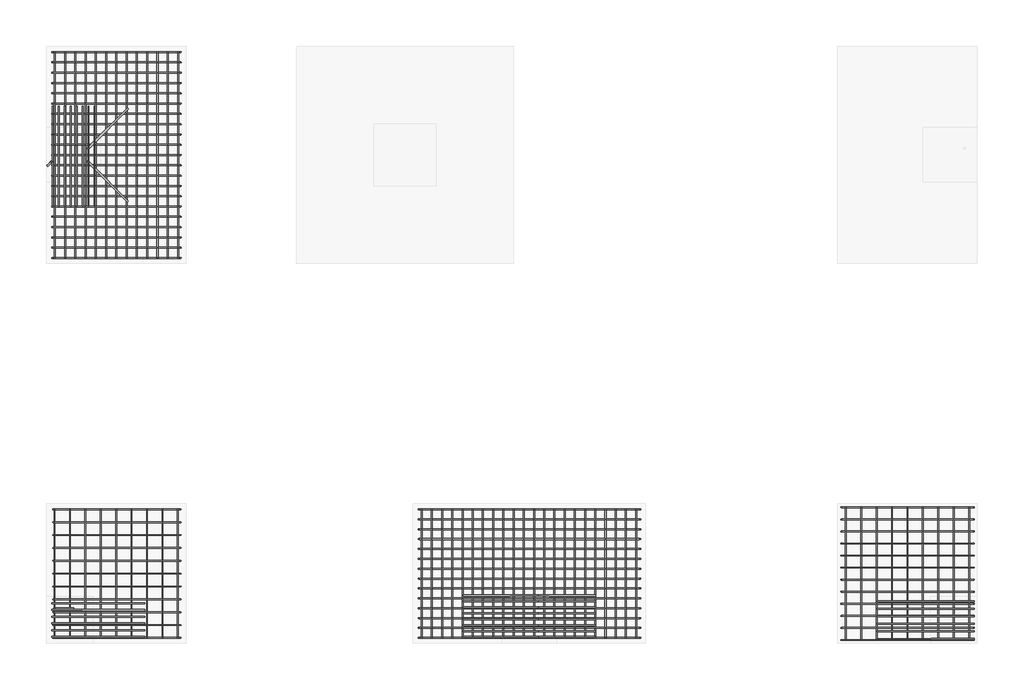
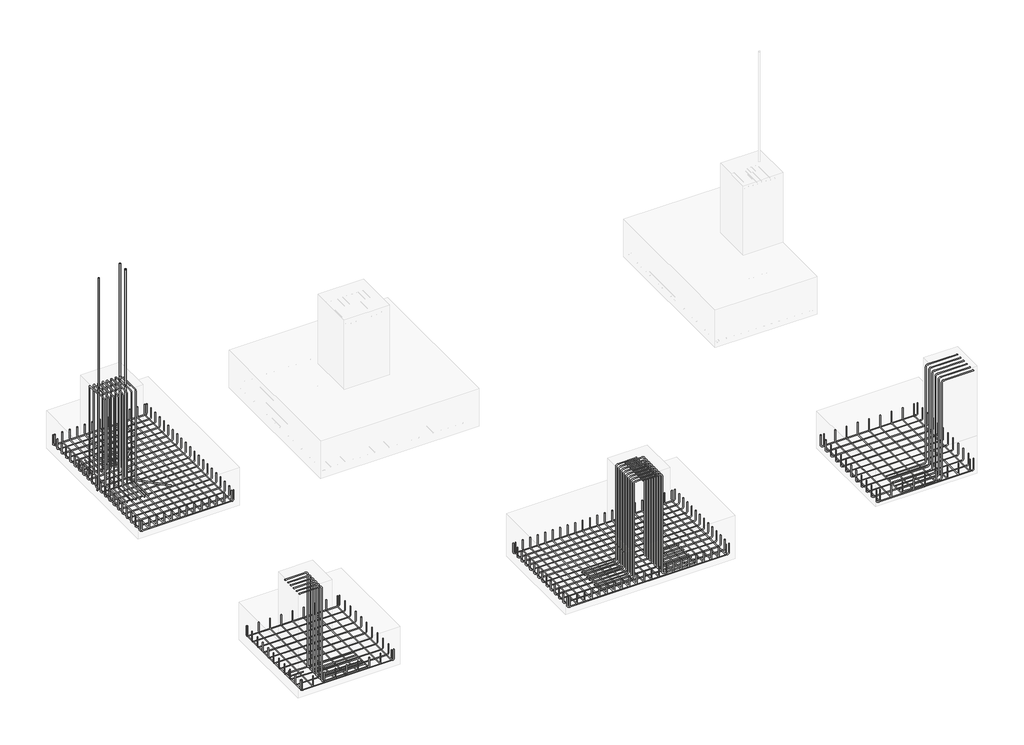
# One storey, part 2 of 6: 18 reinforcing bars.
"""IFC4 building model written with IfcOpenShell, lengths in millimetres."""

from ifc_helpers import new_model, si_unit, point, frame, origin, place, context, project, spatial, polyline, circle_curve, trimmed, segment, composite_curve, source, transform, mapped, element, save
from ifc_brep_helpers import swept_disk

model = new_model("IFC4")

# Units and contexts
model_context = context("Model", 3, world=origin())
ifc_project = project(units=[si_unit("LENGTHUNIT", "METRE", prefix="MILLI")], contexts=[model_context])

# Site, building, storey
site = spatial("IfcSite", under=ifc_project)
building = spatial("IfcBuilding", under=site)
storey = spatial("IfcBuildingStorey", under=building, Elevation=0.0)

# Reinforcing bars
placement = place(None, origin())
reinforcing_bar_shape = source(origin(), model_context, "Body", "SolidModel", [
    swept_disk(composite_curve([segment(polyline([(150339.5463391, -108559.1007776, -331.0), (150339.5463391, -108559.1007776, -459.4)]), True, "CONTINUOUS"), segment(trimmed(circle_curve(frame((150359.5463391, -108559.1007776, -459.4), z_axis=(0.0, -1.0, 0.0), x_axis=(-20.0, 0.0, 0.0)), 20.0), [point((150339.5463391, -108559.1007776, -459.4))], [point((150359.5463391, -108559.1007776, -479.4))], True, "CARTESIAN"), True, "CONTINUOUS"), segment(polyline([(150359.5463391, -108559.1007776, -479.4), (151572.0232069, -108559.1007776, -479.4)]), True, "CONTINUOUS"), segment(trimmed(circle_curve(frame((151572.0232069, -108559.1007776, -459.4), z_axis=(0.0, -1.0, 0.0), x_axis=(0.0, 0.0, -20.0)), 20.0), [point((151572.0232069, -108559.1007776, -479.4))], [point((151592.0232069, -108559.1007776, -459.4))], True, "CARTESIAN"), True, "CONTINUOUS"), segment(polyline([(151592.0232069, -108559.1007776, -459.4), (151592.0232069, -108559.1007776, -331.0)]), True, "CONTINUOUS")], self_intersect=False), 4.0),
])
element("IfcReinforcingBar", 1, at=placement, inside=storey, context=model_context, shape_type="MappedRepresentation", body=[
    mapped(reinforcing_bar_shape, transform((0.0, 0.0, 0.0), x_axis=(1.0, 0.0, 0.0), y_axis=(0.0, 1.0, 0.0), z_axis=(0.0, 0.0, 1.0))),
    mapped(reinforcing_bar_shape, transform((0.0, -126.36, 0.0), x_axis=(1.0, 0.0, 0.0), y_axis=(0.0, 1.0, 0.0), z_axis=(0.0, 0.0, 1.0))),
    mapped(reinforcing_bar_shape, transform((0.0, -252.72, 0.0), x_axis=(1.0, 0.0, 0.0), y_axis=(0.0, 1.0, 0.0), z_axis=(0.0, 0.0, 1.0))),
    mapped(reinforcing_bar_shape, transform((0.0, -379.08, 0.0), x_axis=(1.0, 0.0, 0.0), y_axis=(0.0, 1.0, 0.0), z_axis=(0.0, 0.0, 1.0))),
    mapped(reinforcing_bar_shape, transform((0.0, -505.44, 0.0), x_axis=(1.0, 0.0, 0.0), y_axis=(0.0, 1.0, 0.0), z_axis=(0.0, 0.0, 1.0))),
    mapped(reinforcing_bar_shape, transform((0.0, -631.8, 0.0), x_axis=(1.0, 0.0, 0.0), y_axis=(0.0, 1.0, 0.0), z_axis=(0.0, 0.0, 1.0))),
    mapped(reinforcing_bar_shape, transform((0.0, -758.16, 0.0), x_axis=(1.0, 0.0, 0.0), y_axis=(0.0, 1.0, 0.0), z_axis=(0.0, 0.0, 1.0))),
    mapped(reinforcing_bar_shape, transform((0.0, -884.52, 0.0), x_axis=(1.0, 0.0, 0.0), y_axis=(0.0, 1.0, 0.0), z_axis=(0.0, 0.0, 1.0))),
    mapped(reinforcing_bar_shape, transform((0.0, -1010.88, 0.0), x_axis=(1.0, 0.0, 0.0), y_axis=(0.0, 1.0, 0.0), z_axis=(0.0, 0.0, 1.0))),
    mapped(reinforcing_bar_shape, transform((0.0, -1137.24, 0.0), x_axis=(1.0, 0.0, 0.0), y_axis=(0.0, 1.0, 0.0), z_axis=(0.0, 0.0, 1.0))),
    mapped(reinforcing_bar_shape, transform((0.0, -1263.6, 0.0), x_axis=(1.0, 0.0, 0.0), y_axis=(0.0, 1.0, 0.0), z_axis=(0.0, 0.0, 1.0))),
])
reinforcing_bar_2_shape = source(origin(), model_context, "Body", "SolidModel", [
    swept_disk(composite_curve([segment(polyline([(150352.7854761, -109822.7007776, -331.0), (150352.7854761, -109822.7007776, -459.4)]), True, "CONTINUOUS"), segment(trimmed(circle_curve(frame((150352.7854761, -109802.7007776, -459.4), z_axis=(1.0, 0.0, 0.0), x_axis=(0.0, -20.0, 0.0)), 20.0), [point((150352.7854761, -109822.7007776, -459.4))], [point((150352.7854761, -109802.7007776, -479.4))], True, "CARTESIAN"), True, "CONTINUOUS"), segment(polyline([(150352.7854761, -109802.7007776, -479.4), (150352.7854761, -108579.1007776, -479.4)]), True, "CONTINUOUS"), segment(trimmed(circle_curve(frame((150352.7854761, -108579.1007776, -459.4), z_axis=(1.0, 0.0, 0.0), x_axis=(0.0, 0.0, -20.0)), 20.0), [point((150352.7854761, -108579.1007776, -479.4))], [point((150352.7854761, -108559.1007776, -459.4))], True, "CARTESIAN"), True, "CONTINUOUS"), segment(polyline([(150352.7854761, -108559.1007776, -459.4), (150352.7854761, -108559.1007776, -331.0)]), True, "CONTINUOUS")], self_intersect=False), 4.0),
])
element("IfcReinforcingBar", 2, at=placement, inside=storey, context=model_context, shape_type="MappedRepresentation", body=[
    mapped(reinforcing_bar_2_shape, transform((0.0, 0.0, 0.0), x_axis=(1.0, 0.0, 0.0), y_axis=(0.0, 1.0, 0.0), z_axis=(0.0, 0.0, 1.0))),
    mapped(reinforcing_bar_2_shape, transform((151.3914875, 0.0, 0.0), x_axis=(1.0, 0.0, 0.0), y_axis=(0.0, 1.0, 0.0), z_axis=(0.0, 0.0, 1.0))),
    mapped(reinforcing_bar_2_shape, transform((302.7829749, 0.0, 0.0), x_axis=(1.0, 0.0, 0.0), y_axis=(0.0, 1.0, 0.0), z_axis=(0.0, 0.0, 1.0))),
    mapped(reinforcing_bar_2_shape, transform((454.1744624, 0.0, 0.0), x_axis=(1.0, 0.0, 0.0), y_axis=(0.0, 1.0, 0.0), z_axis=(0.0, 0.0, 1.0))),
    mapped(reinforcing_bar_2_shape, transform((605.5659499, 0.0, 0.0), x_axis=(1.0, 0.0, 0.0), y_axis=(0.0, 1.0, 0.0), z_axis=(0.0, 0.0, 1.0))),
    mapped(reinforcing_bar_2_shape, transform((756.9574374, 0.0, 0.0), x_axis=(1.0, 0.0, 0.0), y_axis=(0.0, 1.0, 0.0), z_axis=(0.0, 0.0, 1.0))),
    mapped(reinforcing_bar_2_shape, transform((908.3489248, 0.0, 0.0), x_axis=(1.0, 0.0, 0.0), y_axis=(0.0, 1.0, 0.0), z_axis=(0.0, 0.0, 1.0))),
    mapped(reinforcing_bar_2_shape, transform((1059.7404123, 0.0, 0.0), x_axis=(1.0, 0.0, 0.0), y_axis=(0.0, 1.0, 0.0), z_axis=(0.0, 0.0, 1.0))),
    mapped(reinforcing_bar_2_shape, transform((1211.1318998, 0.0, 0.0), x_axis=(1.0, 0.0, 0.0), y_axis=(0.0, 1.0, 0.0), z_axis=(0.0, 0.0, 1.0))),
])
reinforcing_bar_3_shape = source(origin(), model_context, "Body", "SolidModel", [
    swept_disk(composite_curve([segment(polyline([(158080.8232069, -108539.1007776, -331.0), (158080.8232069, -108539.1007776, -479.4)]), True, "CONTINUOUS"), segment(trimmed(circle_curve(frame((158100.8232069, -108539.1007776, -479.4), z_axis=(0.0, -1.0, 0.0), x_axis=(-20.0, 0.0, 0.0)), 20.0), [point((158080.8232069, -108539.1007776, -479.4))], [point((158100.8232069, -108539.1007776, -499.4))], True, "CARTESIAN"), True, "CONTINUOUS"), segment(polyline([(158100.8232069, -108539.1007776, -499.4), (159364.4232069, -108539.1007776, -499.4)]), True, "CONTINUOUS"), segment(trimmed(circle_curve(frame((159364.4232069, -108539.1007776, -479.4), z_axis=(0.0, -1.0, 0.0), x_axis=(0.0, 0.0, -20.0)), 20.0), [point((159364.4232069, -108539.1007776, -499.4))], [point((159384.4232069, -108539.1007776, -479.4))], True, "CARTESIAN"), True, "CONTINUOUS"), segment(polyline([(159384.4232069, -108539.1007776, -479.4), (159384.4232069, -108539.1007776, -331.0)]), True, "CONTINUOUS")], self_intersect=False), 4.0),
])
element("IfcReinforcingBar", 3, at=placement, inside=storey, context=model_context, shape_type="MappedRepresentation", body=[
    mapped(reinforcing_bar_3_shape, transform((0.0, 0.0, 0.0), x_axis=(1.0, 0.0, 0.0), y_axis=(0.0, 1.0, 0.0), z_axis=(0.0, 0.0, 1.0))),
    mapped(reinforcing_bar_3_shape, transform((0.0, -118.5090909, 0.0), x_axis=(1.0, 0.0, 0.0), y_axis=(0.0, 1.0, 0.0), z_axis=(0.0, 0.0, 1.0))),
    mapped(reinforcing_bar_3_shape, transform((0.0, -237.0181818, 0.0), x_axis=(1.0, 0.0, 0.0), y_axis=(0.0, 1.0, 0.0), z_axis=(0.0, 0.0, 1.0))),
    mapped(reinforcing_bar_3_shape, transform((0.0, -355.5272727, 0.0), x_axis=(1.0, 0.0, 0.0), y_axis=(0.0, 1.0, 0.0), z_axis=(0.0, 0.0, 1.0))),
    mapped(reinforcing_bar_3_shape, transform((0.0, -474.0363636, 0.0), x_axis=(1.0, 0.0, 0.0), y_axis=(0.0, 1.0, 0.0), z_axis=(0.0, 0.0, 1.0))),
    mapped(reinforcing_bar_3_shape, transform((0.0, -592.5454545, 0.0), x_axis=(1.0, 0.0, 0.0), y_axis=(0.0, 1.0, 0.0), z_axis=(0.0, 0.0, 1.0))),
    mapped(reinforcing_bar_3_shape, transform((0.0, -711.0545455, 0.0), x_axis=(1.0, 0.0, 0.0), y_axis=(0.0, 1.0, 0.0), z_axis=(0.0, 0.0, 1.0))),
    mapped(reinforcing_bar_3_shape, transform((0.0, -829.5636364, 0.0), x_axis=(1.0, 0.0, 0.0), y_axis=(0.0, 1.0, 0.0), z_axis=(0.0, 0.0, 1.0))),
    mapped(reinforcing_bar_3_shape, transform((0.0, -948.0727273, 0.0), x_axis=(1.0, 0.0, 0.0), y_axis=(0.0, 1.0, 0.0), z_axis=(0.0, 0.0, 1.0))),
    mapped(reinforcing_bar_3_shape, transform((0.0, -1066.5818182, 0.0), x_axis=(1.0, 0.0, 0.0), y_axis=(0.0, 1.0, 0.0), z_axis=(0.0, 0.0, 1.0))),
    mapped(reinforcing_bar_3_shape, transform((0.0, -1185.0909091, 0.0), x_axis=(1.0, 0.0, 0.0), y_axis=(0.0, 1.0, 0.0), z_axis=(0.0, 0.0, 1.0))),
    mapped(reinforcing_bar_3_shape, transform((0.0, -1303.6, 0.0), x_axis=(1.0, 0.0, 0.0), y_axis=(0.0, 1.0, 0.0), z_axis=(0.0, 0.0, 1.0))),
])
reinforcing_bar_4_shape = source(origin(), model_context, "Body", "SolidModel", [
    swept_disk(composite_curve([segment(polyline([(158125.1854761, -109842.7007776, -331.0), (158125.1854761, -109842.7007776, -479.4)]), True, "CONTINUOUS"), segment(trimmed(circle_curve(frame((158125.1854761, -109822.7007776, -479.4), z_axis=(1.0, 0.0, 0.0), x_axis=(0.0, -20.0, 0.0)), 20.0), [point((158125.1854761, -109842.7007776, -479.4))], [point((158125.1854761, -109822.7007776, -499.4))], True, "CARTESIAN"), True, "CONTINUOUS"), segment(polyline([(158125.1854761, -109822.7007776, -499.4), (158125.1854761, -108559.1007776, -499.4)]), True, "CONTINUOUS"), segment(trimmed(circle_curve(frame((158125.1854761, -108559.1007776, -479.4), z_axis=(1.0, 0.0, 0.0), x_axis=(0.0, 0.0, -20.0)), 20.0), [point((158125.1854761, -108559.1007776, -499.4))], [point((158125.1854761, -108539.1007776, -479.4))], True, "CARTESIAN"), True, "CONTINUOUS"), segment(polyline([(158125.1854761, -108539.1007776, -479.4), (158125.1854761, -108539.1007776, -331.0)]), True, "CONTINUOUS")], self_intersect=False), 4.0),
])
element("IfcReinforcingBar", 4, at=placement, inside=storey, context=model_context, shape_type="MappedRepresentation", body=[
    mapped(reinforcing_bar_4_shape, transform((0.0, 0.0, 0.0), x_axis=(1.0, 0.0, 0.0), y_axis=(0.0, 1.0, 0.0), z_axis=(0.0, 0.0, 1.0))),
    mapped(reinforcing_bar_4_shape, transform((151.3914875, 0.0, 0.0), x_axis=(1.0, 0.0, 0.0), y_axis=(0.0, 1.0, 0.0), z_axis=(0.0, 0.0, 1.0))),
    mapped(reinforcing_bar_4_shape, transform((302.7829749, 0.0, 0.0), x_axis=(1.0, 0.0, 0.0), y_axis=(0.0, 1.0, 0.0), z_axis=(0.0, 0.0, 1.0))),
    mapped(reinforcing_bar_4_shape, transform((454.1744624, 0.0, 0.0), x_axis=(1.0, 0.0, 0.0), y_axis=(0.0, 1.0, 0.0), z_axis=(0.0, 0.0, 1.0))),
    mapped(reinforcing_bar_4_shape, transform((605.5659499, 0.0, 0.0), x_axis=(1.0, 0.0, 0.0), y_axis=(0.0, 1.0, 0.0), z_axis=(0.0, 0.0, 1.0))),
    mapped(reinforcing_bar_4_shape, transform((756.9574374, 0.0, 0.0), x_axis=(1.0, 0.0, 0.0), y_axis=(0.0, 1.0, 0.0), z_axis=(0.0, 0.0, 1.0))),
    mapped(reinforcing_bar_4_shape, transform((908.3489248, 0.0, 0.0), x_axis=(1.0, 0.0, 0.0), y_axis=(0.0, 1.0, 0.0), z_axis=(0.0, 0.0, 1.0))),
    mapped(reinforcing_bar_4_shape, transform((1059.7404123, 0.0, 0.0), x_axis=(1.0, 0.0, 0.0), y_axis=(0.0, 1.0, 0.0), z_axis=(0.0, 0.0, 1.0))),
    mapped(reinforcing_bar_4_shape, transform((1211.1318998, 0.0, 0.0), x_axis=(1.0, 0.0, 0.0), y_axis=(0.0, 1.0, 0.0), z_axis=(0.0, 0.0, 1.0))),
])
reinforcing_bar_5_shape = source(origin(), model_context, "Body", "SolidModel", [
    swept_disk(composite_curve([segment(polyline([(150329.4309584, -104064.3162805, -331.0), (150329.4309584, -104064.3162805, -453.4)]), True, "CONTINUOUS"), segment(trimmed(circle_curve(frame((150354.4309584, -104064.3162805, -453.4), z_axis=(0.0, -1.0, 0.0), x_axis=(-25.0, 0.0, 0.0)), 25.0), [point((150329.4309584, -104064.3162805, -453.4))], [point((150354.4309584, -104064.3162805, -478.4))], True, "CARTESIAN"), True, "CONTINUOUS"), segment(polyline([(150354.4309584, -104064.3162805, -478.4), (151566.0309584, -104064.3162805, -478.4)]), True, "CONTINUOUS"), segment(trimmed(circle_curve(frame((151566.0309584, -104064.3162805, -453.4), z_axis=(0.0, -1.0, 0.0), x_axis=(0.0, 0.0, -25.0)), 25.0), [point((151566.0309584, -104064.3162805, -478.4))], [point((151591.0309584, -104064.3162805, -453.4))], True, "CARTESIAN"), True, "CONTINUOUS"), segment(polyline([(151591.0309584, -104064.3162805, -453.4), (151591.0309584, -104064.3162805, -331.0)]), True, "CONTINUOUS")], self_intersect=False), 5.0),
])
element("IfcReinforcingBar", 5, at=placement, inside=storey, context=model_context, shape_type="MappedRepresentation", body=[
    mapped(reinforcing_bar_5_shape, transform((0.0, 0.0, 0.0), x_axis=(1.0, 0.0, 0.0), y_axis=(0.0, 1.0, 0.0), z_axis=(0.0, 0.0, 1.0))),
    mapped(reinforcing_bar_5_shape, transform((0.0, -101.18, 0.0), x_axis=(1.0, 0.0, 0.0), y_axis=(0.0, 1.0, 0.0), z_axis=(0.0, 0.0, 1.0))),
    mapped(reinforcing_bar_5_shape, transform((0.0, -202.36, 0.0), x_axis=(1.0, 0.0, 0.0), y_axis=(0.0, 1.0, 0.0), z_axis=(0.0, 0.0, 1.0))),
    mapped(reinforcing_bar_5_shape, transform((0.0, -303.54, 0.0), x_axis=(1.0, 0.0, 0.0), y_axis=(0.0, 1.0, 0.0), z_axis=(0.0, 0.0, 1.0))),
    mapped(reinforcing_bar_5_shape, transform((0.0, -404.72, 0.0), x_axis=(1.0, 0.0, 0.0), y_axis=(0.0, 1.0, 0.0), z_axis=(0.0, 0.0, 1.0))),
    mapped(reinforcing_bar_5_shape, transform((0.0, -505.9, 0.0), x_axis=(1.0, 0.0, 0.0), y_axis=(0.0, 1.0, 0.0), z_axis=(0.0, 0.0, 1.0))),
    mapped(reinforcing_bar_5_shape, transform((0.0, -607.08, 0.0), x_axis=(1.0, 0.0, 0.0), y_axis=(0.0, 1.0, 0.0), z_axis=(0.0, 0.0, 1.0))),
    mapped(reinforcing_bar_5_shape, transform((0.0, -708.26, 0.0), x_axis=(1.0, 0.0, 0.0), y_axis=(0.0, 1.0, 0.0), z_axis=(0.0, 0.0, 1.0))),
    mapped(reinforcing_bar_5_shape, transform((0.0, -809.44, 0.0), x_axis=(1.0, 0.0, 0.0), y_axis=(0.0, 1.0, 0.0), z_axis=(0.0, 0.0, 1.0))),
    mapped(reinforcing_bar_5_shape, transform((0.0, -910.62, 0.0), x_axis=(1.0, 0.0, 0.0), y_axis=(0.0, 1.0, 0.0), z_axis=(0.0, 0.0, 1.0))),
    mapped(reinforcing_bar_5_shape, transform((0.0, -1011.8, 0.0), x_axis=(1.0, 0.0, 0.0), y_axis=(0.0, 1.0, 0.0), z_axis=(0.0, 0.0, 1.0))),
    mapped(reinforcing_bar_5_shape, transform((0.0, -1112.98, 0.0), x_axis=(1.0, 0.0, 0.0), y_axis=(0.0, 1.0, 0.0), z_axis=(0.0, 0.0, 1.0))),
    mapped(reinforcing_bar_5_shape, transform((0.0, -1214.16, 0.0), x_axis=(1.0, 0.0, 0.0), y_axis=(0.0, 1.0, 0.0), z_axis=(0.0, 0.0, 1.0))),
    mapped(reinforcing_bar_5_shape, transform((0.0, -1315.34, 0.0), x_axis=(1.0, 0.0, 0.0), y_axis=(0.0, 1.0, 0.0), z_axis=(0.0, 0.0, 1.0))),
    mapped(reinforcing_bar_5_shape, transform((0.0, -1416.52, 0.0), x_axis=(1.0, 0.0, 0.0), y_axis=(0.0, 1.0, 0.0), z_axis=(0.0, 0.0, 1.0))),
    mapped(reinforcing_bar_5_shape, transform((0.0, -1517.7, 0.0), x_axis=(1.0, 0.0, 0.0), y_axis=(0.0, 1.0, 0.0), z_axis=(0.0, 0.0, 1.0))),
    mapped(reinforcing_bar_5_shape, transform((0.0, -1618.88, 0.0), x_axis=(1.0, 0.0, 0.0), y_axis=(0.0, 1.0, 0.0), z_axis=(0.0, 0.0, 1.0))),
    mapped(reinforcing_bar_5_shape, transform((0.0, -1720.06, 0.0), x_axis=(1.0, 0.0, 0.0), y_axis=(0.0, 1.0, 0.0), z_axis=(0.0, 0.0, 1.0))),
    mapped(reinforcing_bar_5_shape, transform((0.0, -1821.24, 0.0), x_axis=(1.0, 0.0, 0.0), y_axis=(0.0, 1.0, 0.0), z_axis=(0.0, 0.0, 1.0))),
    mapped(reinforcing_bar_5_shape, transform((0.0, -1922.42, 0.0), x_axis=(1.0, 0.0, 0.0), y_axis=(0.0, 1.0, 0.0), z_axis=(0.0, 0.0, 1.0))),
    mapped(reinforcing_bar_5_shape, transform((0.0, -2023.6, 0.0), x_axis=(1.0, 0.0, 0.0), y_axis=(0.0, 1.0, 0.0), z_axis=(0.0, 0.0, 1.0))),
])
reinforcing_bar_6_shape = source(origin(), model_context, "Body", "SolidModel", [
    swept_disk(composite_curve([segment(polyline([(150354.8756407, -106087.9162805, -331.0), (150354.8756407, -106087.9162805, -453.4)]), True, "CONTINUOUS"), segment(trimmed(circle_curve(frame((150354.8756407, -106062.9162805, -453.4), z_axis=(1.0, 0.0, 0.0), x_axis=(0.0, -25.0, 0.0)), 25.0), [point((150354.8756407, -106087.9162805, -453.4))], [point((150354.8756407, -106062.9162805, -478.4))], True, "CARTESIAN"), True, "CONTINUOUS"), segment(polyline([(150354.8756407, -106062.9162805, -478.4), (150354.8756407, -104089.3162805, -478.4)]), True, "CONTINUOUS"), segment(trimmed(circle_curve(frame((150354.8756407, -104089.3162805, -453.4), z_axis=(1.0, 0.0, 0.0), x_axis=(0.0, 0.0, -25.0)), 25.0), [point((150354.8756407, -104089.3162805, -478.4))], [point((150354.8756407, -104064.3162805, -453.4))], True, "CARTESIAN"), True, "CONTINUOUS"), segment(polyline([(150354.8756407, -104064.3162805, -453.4), (150354.8756407, -104064.3162805, -331.0)]), True, "CONTINUOUS")], self_intersect=False), 5.0),
])
element("IfcReinforcingBar", 6, at=placement, inside=storey, context=model_context, shape_type="MappedRepresentation", body=[
    mapped(reinforcing_bar_6_shape, transform((0.0, 0.0, 0.0), x_axis=(1.0, 0.0, 0.0), y_axis=(0.0, 1.0, 0.0), z_axis=(0.0, 0.0, 1.0))),
    mapped(reinforcing_bar_6_shape, transform((100.9434332, 0.0, 0.0), x_axis=(1.0, 0.0, 0.0), y_axis=(0.0, 1.0, 0.0), z_axis=(0.0, 0.0, 1.0))),
    mapped(reinforcing_bar_6_shape, transform((201.8868664, 0.0, 0.0), x_axis=(1.0, 0.0, 0.0), y_axis=(0.0, 1.0, 0.0), z_axis=(0.0, 0.0, 1.0))),
    mapped(reinforcing_bar_6_shape, transform((302.8302996, 0.0, 0.0), x_axis=(1.0, 0.0, 0.0), y_axis=(0.0, 1.0, 0.0), z_axis=(0.0, 0.0, 1.0))),
    mapped(reinforcing_bar_6_shape, transform((403.7737328, 0.0, 0.0), x_axis=(1.0, 0.0, 0.0), y_axis=(0.0, 1.0, 0.0), z_axis=(0.0, 0.0, 1.0))),
    mapped(reinforcing_bar_6_shape, transform((504.717166, 0.0, 0.0), x_axis=(1.0, 0.0, 0.0), y_axis=(0.0, 1.0, 0.0), z_axis=(0.0, 0.0, 1.0))),
    mapped(reinforcing_bar_6_shape, transform((605.6605992, 0.0, 0.0), x_axis=(1.0, 0.0, 0.0), y_axis=(0.0, 1.0, 0.0), z_axis=(0.0, 0.0, 1.0))),
    mapped(reinforcing_bar_6_shape, transform((706.6040324, 0.0, 0.0), x_axis=(1.0, 0.0, 0.0), y_axis=(0.0, 1.0, 0.0), z_axis=(0.0, 0.0, 1.0))),
    mapped(reinforcing_bar_6_shape, transform((807.5474656, 0.0, 0.0), x_axis=(1.0, 0.0, 0.0), y_axis=(0.0, 1.0, 0.0), z_axis=(0.0, 0.0, 1.0))),
    mapped(reinforcing_bar_6_shape, transform((908.4908989, 0.0, 0.0), x_axis=(1.0, 0.0, 0.0), y_axis=(0.0, 1.0, 0.0), z_axis=(0.0, 0.0, 1.0))),
    mapped(reinforcing_bar_6_shape, transform((1009.4343321, 0.0, 0.0), x_axis=(1.0, 0.0, 0.0), y_axis=(0.0, 1.0, 0.0), z_axis=(0.0, 0.0, 1.0))),
    mapped(reinforcing_bar_6_shape, transform((1110.3777653, 0.0, 0.0), x_axis=(1.0, 0.0, 0.0), y_axis=(0.0, 1.0, 0.0), z_axis=(0.0, 0.0, 1.0))),
    mapped(reinforcing_bar_6_shape, transform((1211.3211985, 0.0, 0.0), x_axis=(1.0, 0.0, 0.0), y_axis=(0.0, 1.0, 0.0), z_axis=(0.0, 0.0, 1.0))),
])
reinforcing_bar_7_shape = source(origin(), model_context, "Body", "SolidModel", [
    swept_disk(composite_curve([segment(polyline([(156105.8732069, -109821.7007776, -407.2), (156105.8732069, -109821.7007776, -529.6)]), True, "CONTINUOUS"), segment(trimmed(circle_curve(frame((156080.8732069, -109821.7007776, -529.6), z_axis=(0.0, 1.0, 0.0), x_axis=(25.0, 0.0, 0.0)), 25.0), [point((156105.8732069, -109821.7007776, -529.6))], [point((156080.8732069, -109821.7007776, -554.6))], True, "CARTESIAN"), True, "CONTINUOUS"), segment(polyline([(156080.8732069, -109821.7007776, -554.6), (153954.8732069, -109821.7007776, -554.6)]), True, "CONTINUOUS"), segment(trimmed(circle_curve(frame((153954.8732069, -109821.7007776, -529.6), z_axis=(0.0, 1.0, 0.0), x_axis=(0.0, 0.0, -25.0)), 25.0), [point((153954.8732069, -109821.7007776, -554.6))], [point((153929.8732069, -109821.7007776, -529.6))], True, "CARTESIAN"), True, "CONTINUOUS"), segment(polyline([(153929.8732069, -109821.7007776, -529.6), (153929.8732069, -109821.7007776, -407.2)]), True, "CONTINUOUS")], self_intersect=False), 5.0),
])
element("IfcReinforcingBar", 7, at=placement, inside=storey, context=model_context, shape_type="MappedRepresentation", body=[
    mapped(reinforcing_bar_7_shape, transform((0.0, 0.0, 0.0), x_axis=(1.0, 0.0, 0.0), y_axis=(0.0, 1.0, 0.0), z_axis=(0.0, 0.0, 1.0))),
    mapped(reinforcing_bar_7_shape, transform((0.0, 97.0461538, 0.0), x_axis=(1.0, 0.0, 0.0), y_axis=(0.0, 1.0, 0.0), z_axis=(0.0, 0.0, 1.0))),
    mapped(reinforcing_bar_7_shape, transform((0.0, 194.0923077, 0.0), x_axis=(1.0, 0.0, 0.0), y_axis=(0.0, 1.0, 0.0), z_axis=(0.0, 0.0, 1.0))),
    mapped(reinforcing_bar_7_shape, transform((0.0, 291.1384615, 0.0), x_axis=(1.0, 0.0, 0.0), y_axis=(0.0, 1.0, 0.0), z_axis=(0.0, 0.0, 1.0))),
    mapped(reinforcing_bar_7_shape, transform((0.0, 388.1846154, 0.0), x_axis=(1.0, 0.0, 0.0), y_axis=(0.0, 1.0, 0.0), z_axis=(0.0, 0.0, 1.0))),
    mapped(reinforcing_bar_7_shape, transform((0.0, 485.2307692, 0.0), x_axis=(1.0, 0.0, 0.0), y_axis=(0.0, 1.0, 0.0), z_axis=(0.0, 0.0, 1.0))),
    mapped(reinforcing_bar_7_shape, transform((0.0, 582.2769231, 0.0), x_axis=(1.0, 0.0, 0.0), y_axis=(0.0, 1.0, 0.0), z_axis=(0.0, 0.0, 1.0))),
    mapped(reinforcing_bar_7_shape, transform((0.0, 679.3230769, 0.0), x_axis=(1.0, 0.0, 0.0), y_axis=(0.0, 1.0, 0.0), z_axis=(0.0, 0.0, 1.0))),
    mapped(reinforcing_bar_7_shape, transform((0.0, 776.3692308, 0.0), x_axis=(1.0, 0.0, 0.0), y_axis=(0.0, 1.0, 0.0), z_axis=(0.0, 0.0, 1.0))),
    mapped(reinforcing_bar_7_shape, transform((0.0, 873.4153846, 0.0), x_axis=(1.0, 0.0, 0.0), y_axis=(0.0, 1.0, 0.0), z_axis=(0.0, 0.0, 1.0))),
    mapped(reinforcing_bar_7_shape, transform((0.0, 970.4615385, 0.0), x_axis=(1.0, 0.0, 0.0), y_axis=(0.0, 1.0, 0.0), z_axis=(0.0, 0.0, 1.0))),
    mapped(reinforcing_bar_7_shape, transform((0.0, 1067.5076923, 0.0), x_axis=(1.0, 0.0, 0.0), y_axis=(0.0, 1.0, 0.0), z_axis=(0.0, 0.0, 1.0))),
    mapped(reinforcing_bar_7_shape, transform((0.0, 1164.5538462, 0.0), x_axis=(1.0, 0.0, 0.0), y_axis=(0.0, 1.0, 0.0), z_axis=(0.0, 0.0, 1.0))),
    mapped(reinforcing_bar_7_shape, transform((0.0, 1261.6, 0.0), x_axis=(1.0, 0.0, 0.0), y_axis=(0.0, 1.0, 0.0), z_axis=(0.0, 0.0, 1.0))),
])
reinforcing_bar_8_shape = source(origin(), model_context, "Body", "SolidModel", [
    swept_disk(composite_curve([segment(polyline([(156065.6929913, -108560.1007776, -407.2), (156065.6929913, -108560.1007776, -529.6)]), True, "CONTINUOUS"), segment(trimmed(circle_curve(frame((156065.6929913, -108585.1007776, -529.6), z_axis=(-1.0, 0.0, 0.0), x_axis=(0.0, 25.0, 0.0)), 25.0), [point((156065.6929913, -108560.1007776, -529.6))], [point((156065.6929913, -108585.1007776, -554.6))], True, "CARTESIAN"), True, "CONTINUOUS"), segment(polyline([(156065.6929913, -108585.1007776, -554.6), (156065.6929913, -109796.7007776, -554.6)]), True, "CONTINUOUS"), segment(trimmed(circle_curve(frame((156065.6929913, -109796.7007776, -529.6), z_axis=(-1.0, 0.0, 0.0), x_axis=(0.0, 0.0, -25.0)), 25.0), [point((156065.6929913, -109796.7007776, -554.6))], [point((156065.6929913, -109821.7007776, -529.6))], True, "CARTESIAN"), True, "CONTINUOUS"), segment(polyline([(156065.6929913, -109821.7007776, -529.6), (156065.6929913, -109821.7007776, -407.2)]), True, "CONTINUOUS")], self_intersect=False), 5.0),
])
element("IfcReinforcingBar", 8, at=placement, inside=storey, context=model_context, shape_type="MappedRepresentation", body=[
    mapped(reinforcing_bar_8_shape, transform((0.0, 0.0, 0.0), x_axis=(1.0, 0.0, 0.0), y_axis=(0.0, 1.0, 0.0), z_axis=(0.0, 0.0, 1.0))),
    mapped(reinforcing_bar_8_shape, transform((-100.2961254, 0.0, 0.0), x_axis=(1.0, 0.0, 0.0), y_axis=(0.0, 1.0, 0.0), z_axis=(0.0, 0.0, 1.0))),
    mapped(reinforcing_bar_8_shape, transform((-200.5922507, 0.0, 0.0), x_axis=(1.0, 0.0, 0.0), y_axis=(0.0, 1.0, 0.0), z_axis=(0.0, 0.0, 1.0))),
    mapped(reinforcing_bar_8_shape, transform((-300.8883761, 0.0, 0.0), x_axis=(1.0, 0.0, 0.0), y_axis=(0.0, 1.0, 0.0), z_axis=(0.0, 0.0, 1.0))),
    mapped(reinforcing_bar_8_shape, transform((-401.1845015, 0.0, 0.0), x_axis=(1.0, 0.0, 0.0), y_axis=(0.0, 1.0, 0.0), z_axis=(0.0, 0.0, 1.0))),
    mapped(reinforcing_bar_8_shape, transform((-501.4806268, 0.0, 0.0), x_axis=(1.0, 0.0, 0.0), y_axis=(0.0, 1.0, 0.0), z_axis=(0.0, 0.0, 1.0))),
    mapped(reinforcing_bar_8_shape, transform((-601.7767522, 0.0, 0.0), x_axis=(1.0, 0.0, 0.0), y_axis=(0.0, 1.0, 0.0), z_axis=(0.0, 0.0, 1.0))),
    mapped(reinforcing_bar_8_shape, transform((-702.0728776, 0.0, 0.0), x_axis=(1.0, 0.0, 0.0), y_axis=(0.0, 1.0, 0.0), z_axis=(0.0, 0.0, 1.0))),
    mapped(reinforcing_bar_8_shape, transform((-802.3690029, 0.0, 0.0), x_axis=(1.0, 0.0, 0.0), y_axis=(0.0, 1.0, 0.0), z_axis=(0.0, 0.0, 1.0))),
    mapped(reinforcing_bar_8_shape, transform((-902.6651283, 0.0, 0.0), x_axis=(1.0, 0.0, 0.0), y_axis=(0.0, 1.0, 0.0), z_axis=(0.0, 0.0, 1.0))),
    mapped(reinforcing_bar_8_shape, transform((-1002.9612537, 0.0, 0.0), x_axis=(1.0, 0.0, 0.0), y_axis=(0.0, 1.0, 0.0), z_axis=(0.0, 0.0, 1.0))),
    mapped(reinforcing_bar_8_shape, transform((-1103.257379, 0.0, 0.0), x_axis=(1.0, 0.0, 0.0), y_axis=(0.0, 1.0, 0.0), z_axis=(0.0, 0.0, 1.0))),
    mapped(reinforcing_bar_8_shape, transform((-1203.5535044, 0.0, 0.0), x_axis=(1.0, 0.0, 0.0), y_axis=(0.0, 1.0, 0.0), z_axis=(0.0, 0.0, 1.0))),
    mapped(reinforcing_bar_8_shape, transform((-1303.8496298, 0.0, 0.0), x_axis=(1.0, 0.0, 0.0), y_axis=(0.0, 1.0, 0.0), z_axis=(0.0, 0.0, 1.0))),
    mapped(reinforcing_bar_8_shape, transform((-1404.1457551, 0.0, 0.0), x_axis=(1.0, 0.0, 0.0), y_axis=(0.0, 1.0, 0.0), z_axis=(0.0, 0.0, 1.0))),
    mapped(reinforcing_bar_8_shape, transform((-1504.4418805, 0.0, 0.0), x_axis=(1.0, 0.0, 0.0), y_axis=(0.0, 1.0, 0.0), z_axis=(0.0, 0.0, 1.0))),
    mapped(reinforcing_bar_8_shape, transform((-1604.7380059, 0.0, 0.0), x_axis=(1.0, 0.0, 0.0), y_axis=(0.0, 1.0, 0.0), z_axis=(0.0, 0.0, 1.0))),
    mapped(reinforcing_bar_8_shape, transform((-1705.0341312, 0.0, 0.0), x_axis=(1.0, 0.0, 0.0), y_axis=(0.0, 1.0, 0.0), z_axis=(0.0, 0.0, 1.0))),
    mapped(reinforcing_bar_8_shape, transform((-1805.3302566, 0.0, 0.0), x_axis=(1.0, 0.0, 0.0), y_axis=(0.0, 1.0, 0.0), z_axis=(0.0, 0.0, 1.0))),
    mapped(reinforcing_bar_8_shape, transform((-1905.626382, 0.0, 0.0), x_axis=(1.0, 0.0, 0.0), y_axis=(0.0, 1.0, 0.0), z_axis=(0.0, 0.0, 1.0))),
    mapped(reinforcing_bar_8_shape, transform((-2005.9225073, 0.0, 0.0), x_axis=(1.0, 0.0, 0.0), y_axis=(0.0, 1.0, 0.0), z_axis=(0.0, 0.0, 1.0))),
    mapped(reinforcing_bar_8_shape, transform((-2106.2186327, 0.0, 0.0), x_axis=(1.0, 0.0, 0.0), y_axis=(0.0, 1.0, 0.0), z_axis=(0.0, 0.0, 1.0))),
])
reinforcing_bar_9_shape = source(origin(), model_context, "Body", "SolidModel", [
    swept_disk(composite_curve([segment(polyline([(150324.4232069, -109813.7007776, 895.3671896), (150604.2232069, -109813.7007776, 895.3671896)]), True, "CONTINUOUS"), segment(trimmed(circle_curve(frame((150604.2232069, -109813.7007776, 870.3671896), z_axis=(0.0, 1.0, 0.0), x_axis=(0.0, 0.0, 25.0)), 25.0), [point((150604.2232069, -109813.7007776, 895.3671896))], [point((150629.2232069, -109813.7007776, 870.3671896))], True, "CARTESIAN"), True, "CONTINUOUS"), segment(polyline([(150629.2232069, -109813.7007776, 870.3671896), (150629.2232069, -109813.7007776, -435.3654732)]), True, "CONTINUOUS"), segment(trimmed(circle_curve(frame((150654.2232069, -109813.7007776, -435.3654732), z_axis=(0.0, -1.0, 0.0), x_axis=(-25.0, 0.0, 0.0)), 25.0), [point((150629.2232069, -109813.7007776, -435.3654732))], [point((150654.2232069, -109813.7007776, -460.3654732))], True, "CARTESIAN"), True, "CONTINUOUS"), segment(polyline([(150654.2232069, -109813.7007776, -460.3654732), (151238.8232069, -109813.7007776, -460.3654732)]), True, "CONTINUOUS")], self_intersect=False), 5.0),
])
element("IfcReinforcingBar", 9, at=placement, inside=storey, context=model_context, shape_type="MappedRepresentation", body=[
    mapped(reinforcing_bar_9_shape, transform((0.0, 0.0, 0.0), x_axis=(1.0, 0.0, 0.0), y_axis=(0.0, 1.0, 0.0), z_axis=(0.0, 0.0, 1.0))),
    mapped(reinforcing_bar_9_shape, transform((0.0, 66.24, 0.0), x_axis=(1.0, 0.0, 0.0), y_axis=(0.0, 1.0, 0.0), z_axis=(0.0, 0.0, 1.0))),
    mapped(reinforcing_bar_9_shape, transform((0.0, 132.48, 0.0), x_axis=(1.0, 0.0, 0.0), y_axis=(0.0, 1.0, 0.0), z_axis=(0.0, 0.0, 1.0))),
    mapped(reinforcing_bar_9_shape, transform((0.0, 198.72, 0.0), x_axis=(1.0, 0.0, 0.0), y_axis=(0.0, 1.0, 0.0), z_axis=(0.0, 0.0, 1.0))),
    mapped(reinforcing_bar_9_shape, transform((0.0, 264.96, 0.0), x_axis=(1.0, 0.0, 0.0), y_axis=(0.0, 1.0, 0.0), z_axis=(0.0, 0.0, 1.0))),
    mapped(reinforcing_bar_9_shape, transform((0.0, 331.2, 0.0), x_axis=(1.0, 0.0, 0.0), y_axis=(0.0, 1.0, 0.0), z_axis=(0.0, 0.0, 1.0))),
])
element("IfcReinforcingBar", 10, at=placement, inside=storey, context=model_context, shape_type="SolidModel", body=[
    swept_disk(composite_curve([segment(polyline([(150541.1232069, -109530.0339158, -462.4652155), (150369.6846071, -109530.0339158, -462.4652155)]), True, "CONTINUOUS"), segment(trimmed(circle_curve(frame((150369.6846071, -109530.0339158, -442.4652155), z_axis=(0.0, 1.0, 0.0), x_axis=(0.0, 0.0, -20.0)), 20.0), [point((150369.6846071, -109530.0339158, -462.4652155))], [point((150349.6846071, -109530.0339158, -442.4652155))], True, "CARTESIAN"), True, "CONTINUOUS"), segment(polyline([(150349.6846071, -109530.0339158, -442.4652155), (150349.6846071, -109530.0339158, -382.8549127)]), True, "CONTINUOUS")], self_intersect=False), 4.0),
])
reinforcing_bar_10_shape = source(origin(), model_context, "Body", "SolidModel", [
    swept_disk(composite_curve([segment(polyline([(150336.4232069, -104983.5351466, 899.6018913), (150336.4232069, -105252.1507776, 899.6018913)]), True, "CONTINUOUS"), segment(trimmed(circle_curve(frame((150336.4232069, -105252.1507776, 879.6018913), z_axis=(1.0, 0.0, 0.0), x_axis=(0.0, 0.0, 20.0)), 20.0), [point((150336.4232069, -105252.1507776, 899.6018913))], [point((150336.4232069, -105272.1507776, 879.6018913))], True, "CARTESIAN"), True, "CONTINUOUS"), segment(polyline([(150336.4232069, -105272.1507776, 879.6018913), (150336.4232069, -105272.1507776, -399.7898753)]), True, "CONTINUOUS"), segment(trimmed(circle_curve(frame((150336.4232069, -105292.1507776, -399.7898753), z_axis=(-1.0, 0.0, 0.0), x_axis=(0.0, 20.0, 0.0)), 20.0), [point((150336.4232069, -105272.1507776, -399.7898753))], [point((150336.4232069, -105292.1507776, -419.7898753))], True, "CARTESIAN"), True, "CONTINUOUS"), segment(polyline([(150336.4232069, -105292.1507776, -419.7898753), (150336.4232069, -105576.9507776, -419.7898753)]), True, "CONTINUOUS")], self_intersect=False), 4.0),
])
element("IfcReinforcingBar", 11, at=placement, inside=storey, context=model_context, shape_type="MappedRepresentation", body=[
    mapped(reinforcing_bar_10_shape, transform((0.0, 0.0, 0.0), x_axis=(1.0, 0.0, 0.0), y_axis=(0.0, 1.0, 0.0), z_axis=(0.0, 0.0, 1.0))),
    mapped(reinforcing_bar_10_shape, transform((58.4857143, 0.0, 0.0), x_axis=(1.0, 0.0, 0.0), y_axis=(0.0, 1.0, 0.0), z_axis=(0.0, 0.0, 1.0))),
    mapped(reinforcing_bar_10_shape, transform((116.9714286, 0.0, 0.0), x_axis=(1.0, 0.0, 0.0), y_axis=(0.0, 1.0, 0.0), z_axis=(0.0, 0.0, 1.0))),
    mapped(reinforcing_bar_10_shape, transform((175.4571429, 0.0, 0.0), x_axis=(1.0, 0.0, 0.0), y_axis=(0.0, 1.0, 0.0), z_axis=(0.0, 0.0, 1.0))),
    mapped(reinforcing_bar_10_shape, transform((233.9428571, 0.0, 0.0), x_axis=(1.0, 0.0, 0.0), y_axis=(0.0, 1.0, 0.0), z_axis=(0.0, 0.0, 1.0))),
    mapped(reinforcing_bar_10_shape, transform((292.4285714, 0.0, 0.0), x_axis=(1.0, 0.0, 0.0), y_axis=(0.0, 1.0, 0.0), z_axis=(0.0, 0.0, 1.0))),
    mapped(reinforcing_bar_10_shape, transform((350.9142857, 0.0, 0.0), x_axis=(1.0, 0.0, 0.0), y_axis=(0.0, 1.0, 0.0), z_axis=(0.0, 0.0, 1.0))),
    mapped(reinforcing_bar_10_shape, transform((409.4, 0.0, 0.0), x_axis=(1.0, 0.0, 0.0), y_axis=(0.0, 1.0, 0.0), z_axis=(0.0, 0.0, 1.0))),
])
reinforcing_bar_11_shape = source(origin(), model_context, "Body", "SolidModel", [
    swept_disk(composite_curve([segment(polyline([(150745.8232069, -105135.8908057, 877.0190747), (150745.8232069, -104920.9408057, 877.0190747)]), True, "CONTINUOUS"), segment(trimmed(circle_curve(frame((150745.8232069, -104920.9408057, 857.0190747), z_axis=(-1.0, 0.0, 0.0), x_axis=(0.0, 0.0, 20.0)), 20.0), [point((150745.8232069, -104920.9408057, 877.0190747))], [point((150745.8232069, -104900.9408057, 857.0190747))], True, "CARTESIAN"), True, "CONTINUOUS"), segment(polyline([(150745.8232069, -104900.9408057, 857.0190747), (150745.8232069, -104900.9408057, -392.0309253)]), True, "CONTINUOUS"), segment(trimmed(circle_curve(frame((150745.8232069, -104880.9408057, -392.0309253), z_axis=(1.0, 0.0, 0.0), x_axis=(0.0, -20.0, 0.0)), 20.0), [point((150745.8232069, -104900.9408057, -392.0309253))], [point((150745.8232069, -104880.9408057, -412.0309253))], True, "CARTESIAN"), True, "CONTINUOUS"), segment(polyline([(150745.8232069, -104880.9408057, -412.0309253), (150745.8232069, -104596.1408057, -412.0309253)]), True, "CONTINUOUS")], self_intersect=False), 4.0),
])
element("IfcReinforcingBar", 12, at=placement, inside=storey, context=model_context, shape_type="MappedRepresentation", body=[
    mapped(reinforcing_bar_11_shape, transform((0.0, 0.0, 0.0), x_axis=(1.0, 0.0, 0.0), y_axis=(0.0, 1.0, 0.0), z_axis=(0.0, 0.0, 1.0))),
    mapped(reinforcing_bar_11_shape, transform((-58.4857143, 0.0, 0.0), x_axis=(1.0, 0.0, 0.0), y_axis=(0.0, 1.0, 0.0), z_axis=(0.0, 0.0, 1.0))),
    mapped(reinforcing_bar_11_shape, transform((-116.9714286, 0.0, 0.0), x_axis=(1.0, 0.0, 0.0), y_axis=(0.0, 1.0, 0.0), z_axis=(0.0, 0.0, 1.0))),
    mapped(reinforcing_bar_11_shape, transform((-175.4571429, 0.0, 0.0), x_axis=(1.0, 0.0, 0.0), y_axis=(0.0, 1.0, 0.0), z_axis=(0.0, 0.0, 1.0))),
    mapped(reinforcing_bar_11_shape, transform((-233.9428571, 0.0, 0.0), x_axis=(1.0, 0.0, 0.0), y_axis=(0.0, 1.0, 0.0), z_axis=(0.0, 0.0, 1.0))),
    mapped(reinforcing_bar_11_shape, transform((-292.4285714, 0.0, 0.0), x_axis=(1.0, 0.0, 0.0), y_axis=(0.0, 1.0, 0.0), z_axis=(0.0, 0.0, 1.0))),
    mapped(reinforcing_bar_11_shape, transform((-350.9142857, 0.0, 0.0), x_axis=(1.0, 0.0, 0.0), y_axis=(0.0, 1.0, 0.0), z_axis=(0.0, 0.0, 1.0))),
    mapped(reinforcing_bar_11_shape, transform((-409.4, 0.0, 0.0), x_axis=(1.0, 0.0, 0.0), y_axis=(0.0, 1.0, 0.0), z_axis=(0.0, 0.0, 1.0))),
])
reinforcing_bar_12_shape = source(origin(), model_context, "Body", "SolidModel", [
    swept_disk(composite_curve([segment(polyline([(155102.7977208, -109406.3007776, 911.8751366), (154851.8732069, -109406.3007776, 911.8751366)]), True, "CONTINUOUS"), segment(trimmed(circle_curve(frame((154851.8732069, -109406.3007776, 886.8751366), z_axis=(0.0, -1.0, 0.0), x_axis=(0.0, 0.0, 25.0)), 25.0), [point((154851.8732069, -109406.3007776, 911.8751366))], [point((154826.8732069, -109406.3007776, 886.8751366))], True, "CARTESIAN"), True, "CONTINUOUS"), segment(polyline([(154826.8732069, -109406.3007776, 886.8751366), (154826.8732069, -109406.3007776, -434.7248634)]), True, "CONTINUOUS"), segment(trimmed(circle_curve(frame((154801.8732069, -109406.3007776, -434.7248634), z_axis=(0.0, 1.0, 0.0), x_axis=(25.0, 0.0, 0.0)), 25.0), [point((154826.8732069, -109406.3007776, -434.7248634))], [point((154801.8732069, -109406.3007776, -459.7248634))], True, "CARTESIAN"), True, "CONTINUOUS"), segment(polyline([(154801.8732069, -109406.3007776, -459.7248634), (154366.1977208, -109406.3007776, -459.7248634)]), True, "CONTINUOUS")], self_intersect=False), 5.0),
])
element("IfcReinforcingBar", 13, at=placement, inside=storey, context=model_context, shape_type="MappedRepresentation", body=[
    mapped(reinforcing_bar_12_shape, transform((0.0, 0.0, 0.0), x_axis=(1.0, 0.0, 0.0), y_axis=(0.0, 1.0, 0.0), z_axis=(0.0, 0.0, 1.0))),
    mapped(reinforcing_bar_12_shape, transform((0.0, -58.2, 0.0), x_axis=(1.0, 0.0, 0.0), y_axis=(0.0, 1.0, 0.0), z_axis=(0.0, 0.0, 1.0))),
    mapped(reinforcing_bar_12_shape, transform((0.0, -116.4, 0.0), x_axis=(1.0, 0.0, 0.0), y_axis=(0.0, 1.0, 0.0), z_axis=(0.0, 0.0, 1.0))),
    mapped(reinforcing_bar_12_shape, transform((0.0, -174.6, 0.0), x_axis=(1.0, 0.0, 0.0), y_axis=(0.0, 1.0, 0.0), z_axis=(0.0, 0.0, 1.0))),
    mapped(reinforcing_bar_12_shape, transform((0.0, -232.8, 0.0), x_axis=(1.0, 0.0, 0.0), y_axis=(0.0, 1.0, 0.0), z_axis=(0.0, 0.0, 1.0))),
    mapped(reinforcing_bar_12_shape, transform((0.0, -291.0, 0.0), x_axis=(1.0, 0.0, 0.0), y_axis=(0.0, 1.0, 0.0), z_axis=(0.0, 0.0, 1.0))),
    mapped(reinforcing_bar_12_shape, transform((0.0, -349.2, 0.0), x_axis=(1.0, 0.0, 0.0), y_axis=(0.0, 1.0, 0.0), z_axis=(0.0, 0.0, 1.0))),
    mapped(reinforcing_bar_12_shape, transform((0.0, -407.4, 0.0), x_axis=(1.0, 0.0, 0.0), y_axis=(0.0, 1.0, 0.0), z_axis=(0.0, 0.0, 1.0))),
])
reinforcing_bar_13_shape = source(origin(), model_context, "Body", "SolidModel", [
    swept_disk(composite_curve([segment(polyline([(154949.3074059, -109813.7007776, 888.8193095), (155184.6574059, -109813.7007776, 888.8193095)]), True, "CONTINUOUS"), segment(trimmed(circle_curve(frame((155184.6574059, -109813.7007776, 863.8193095), z_axis=(0.0, 1.0, 0.0), x_axis=(0.0, 0.0, 25.0)), 25.0), [point((155184.6574059, -109813.7007776, 888.8193095))], [point((155209.6574059, -109813.7007776, 863.8193095))], True, "CARTESIAN"), True, "CONTINUOUS"), segment(polyline([(155209.6574059, -109813.7007776, 863.8193095), (155209.6574059, -109813.7007776, -499.7062218)]), True, "CONTINUOUS"), segment(trimmed(circle_curve(frame((155234.6574059, -109813.7007776, -499.7062218), z_axis=(0.0, -1.0, 0.0), x_axis=(-25.0, 0.0, 0.0)), 25.0), [point((155209.6574059, -109813.7007776, -499.7062218))], [point((155234.6574059, -109813.7007776, -524.7062218))], True, "CARTESIAN"), True, "CONTINUOUS"), segment(polyline([(155234.6574059, -109813.7007776, -524.7062218), (155666.8574059, -109813.7007776, -524.7062218)]), True, "CONTINUOUS")], self_intersect=False), 5.0),
])
element("IfcReinforcingBar", 14, at=placement, inside=storey, context=model_context, shape_type="MappedRepresentation", body=[
    mapped(reinforcing_bar_13_shape, transform((0.0, 0.0, 0.0), x_axis=(1.0, 0.0, 0.0), y_axis=(0.0, 1.0, 0.0), z_axis=(0.0, 0.0, 1.0))),
    mapped(reinforcing_bar_13_shape, transform((0.0, 58.2, 0.0), x_axis=(1.0, 0.0, 0.0), y_axis=(0.0, 1.0, 0.0), z_axis=(0.0, 0.0, 1.0))),
    mapped(reinforcing_bar_13_shape, transform((0.0, 116.4, 0.0), x_axis=(1.0, 0.0, 0.0), y_axis=(0.0, 1.0, 0.0), z_axis=(0.0, 0.0, 1.0))),
    mapped(reinforcing_bar_13_shape, transform((0.0, 174.6, 0.0), x_axis=(1.0, 0.0, 0.0), y_axis=(0.0, 1.0, 0.0), z_axis=(0.0, 0.0, 1.0))),
    mapped(reinforcing_bar_13_shape, transform((0.0, 232.8, 0.0), x_axis=(1.0, 0.0, 0.0), y_axis=(0.0, 1.0, 0.0), z_axis=(0.0, 0.0, 1.0))),
    mapped(reinforcing_bar_13_shape, transform((0.0, 291.0, 0.0), x_axis=(1.0, 0.0, 0.0), y_axis=(0.0, 1.0, 0.0), z_axis=(0.0, 0.0, 1.0))),
    mapped(reinforcing_bar_13_shape, transform((0.0, 349.2, 0.0), x_axis=(1.0, 0.0, 0.0), y_axis=(0.0, 1.0, 0.0), z_axis=(0.0, 0.0, 1.0))),
    mapped(reinforcing_bar_13_shape, transform((0.0, 407.4, 0.0), x_axis=(1.0, 0.0, 0.0), y_axis=(0.0, 1.0, 0.0), z_axis=(0.0, 0.0, 1.0))),
])
element("IfcReinforcingBar", 15, at=placement, inside=storey, context=model_context, shape_type="SolidModel", body=[
    swept_disk(composite_curve([segment(polyline([(150322.8982069, -105141.9257776, 2557.2891341), (150322.8982069, -105141.9257776, -382.0926147)]), True, "CONTINUOUS"), segment(trimmed(circle_curve(frame((150294.6139357, -105170.2100488, -382.0926147), z_axis=(-0.70710678118641, 0.707106781186685, 0.0), x_axis=(28.284271199983777, 28.28427119999833, 0.0)), 40.0), [point((150322.8982069, -105141.9257776, -382.0926147))], [point((150294.6139357, -105170.2100488, -422.0926147))], True, "CARTESIAN"), True, "CONTINUOUS"), segment(polyline([(150294.6139357, -105170.2100488, -422.0926147), (150282.8106273, -105182.0133572, -422.0926147)]), True, "CONTINUOUS")], self_intersect=False), 8.0),
])
element("IfcReinforcingBar", 16, at=placement, inside=storey, context=model_context, shape_type="SolidModel", body=[
    swept_disk(composite_curve([segment(polyline([(150683.2800612, -105142.0576318, 2557.2891341), (150683.2800612, -105142.0576318, -382.0926147)]), True, "CONTINUOUS"), segment(trimmed(circle_curve(frame((150711.5643324, -105170.3419031, -382.0926147), z_axis=(-0.7071067811865172, -0.7071067811865779, 0.0), x_axis=(-28.28427120001288, 28.28427129999909, 0.0)), 40.0), [point((150683.2800612, -105142.0576318, -382.0926147))], [point((150711.5643324, -105170.3419031, -422.0926147))], True, "CARTESIAN"), True, "CONTINUOUS"), segment(polyline([(150711.5643324, -105170.3419031, -422.0926147), (151073.421381, -105532.1989517, -422.0926147)]), True, "CONTINUOUS")], self_intersect=False), 8.0),
])
element("IfcReinforcingBar", 17, at=placement, inside=storey, context=model_context, shape_type="SolidModel", body=[
    swept_disk(composite_curve([segment(polyline([(150683.2800612, -105010.1439233, 2557.2891341), (150683.2800612, -105010.1439233, -382.0926147)]), True, "CONTINUOUS"), segment(trimmed(circle_curve(frame((150711.5643324, -104981.8596521, -382.0926147), z_axis=(0.70710678118641, -0.707106781186685, 0.0), x_axis=(-28.28427120001288, -28.28427119999833, 0.0)), 40.0), [point((150683.2800612, -105010.1439233, -382.0926147))], [point((150711.5643324, -104981.8596521, -422.0926147))], True, "CARTESIAN"), True, "CONTINUOUS"), segment(polyline([(150711.5643324, -104981.8596521, -422.0926147), (151073.421381, -104620.0026035, -422.0926147)]), True, "CONTINUOUS")], self_intersect=False), 8.0),
])
reinforcing_bar_14_shape = source(origin(), model_context, "Body", "SolidModel", [
    swept_disk(composite_curve([segment(polyline([(159388.4232069, -109833.7007776, 915.3671896), (158988.7353832, -109833.7007776, 915.3671896)]), True, "CONTINUOUS"), segment(trimmed(circle_curve(frame((158988.7353832, -109833.7007776, 890.3671896), z_axis=(0.0, -1.0, 0.0), x_axis=(0.0, 0.0, 25.0)), 25.0), [point((158988.7353832, -109833.7007776, 915.3671896))], [point((158963.7353832, -109833.7007776, 890.3671896))], True, "CARTESIAN"), True, "CONTINUOUS"), segment(polyline([(158963.7353832, -109833.7007776, 890.3671896), (158963.7353832, -109833.7007776, -455.3654732)]), True, "CONTINUOUS"), segment(trimmed(circle_curve(frame((158938.7353832, -109833.7007776, -455.3654732), z_axis=(0.0, 1.0, 0.0), x_axis=(25.0, 0.0, 0.0)), 25.0), [point((158963.7353832, -109833.7007776, -455.3654732))], [point((158938.7353832, -109833.7007776, -480.3654732))], True, "CARTESIAN"), True, "CONTINUOUS"), segment(polyline([(158938.7353832, -109833.7007776, -480.3654732), (158434.0232069, -109833.7007776, -480.3654732)]), True, "CONTINUOUS")], self_intersect=False), 5.0),
])
element("IfcReinforcingBar", 18, at=placement, inside=storey, context=model_context, shape_type="MappedRepresentation", body=[
    mapped(reinforcing_bar_14_shape, transform((0.0, 0.0, 0.0), x_axis=(1.0, 0.0, 0.0), y_axis=(0.0, 1.0, 0.0), z_axis=(0.0, 0.0, 1.0))),
    mapped(reinforcing_bar_14_shape, transform((0.0, 74.24, 0.0), x_axis=(1.0, 0.0, 0.0), y_axis=(0.0, 1.0, 0.0), z_axis=(0.0, 0.0, 1.0))),
    mapped(reinforcing_bar_14_shape, transform((0.0, 148.48, 0.0), x_axis=(1.0, 0.0, 0.0), y_axis=(0.0, 1.0, 0.0), z_axis=(0.0, 0.0, 1.0))),
    mapped(reinforcing_bar_14_shape, transform((0.0, 222.72, 0.0), x_axis=(1.0, 0.0, 0.0), y_axis=(0.0, 1.0, 0.0), z_axis=(0.0, 0.0, 1.0))),
    mapped(reinforcing_bar_14_shape, transform((0.0, 296.96, 0.0), x_axis=(1.0, 0.0, 0.0), y_axis=(0.0, 1.0, 0.0), z_axis=(0.0, 0.0, 1.0))),
    mapped(reinforcing_bar_14_shape, transform((0.0, 371.2, 0.0), x_axis=(1.0, 0.0, 0.0), y_axis=(0.0, 1.0, 0.0), z_axis=(0.0, 0.0, 1.0))),
])

save(model, "model.ifc")

# Revit data of these elements
# Elements 1, 2, 3, 4, 5, 6, 7, 8, 9, 10, 11, 12, 13, 14, 15, 16, 17, 18 (IfcReinforcingBar)
#   Phase Created = New Construction
